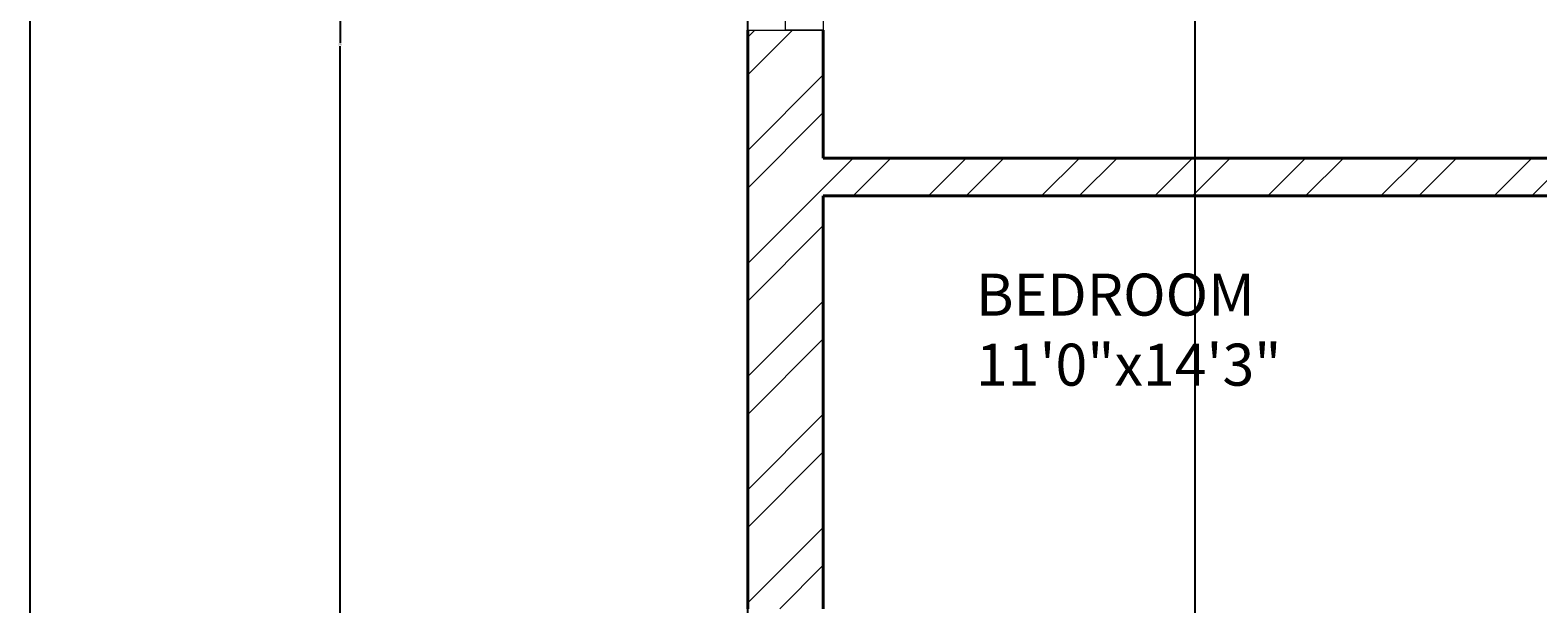
# Model space of a CAD drawing. Units: inches. Extents: x 1601 to 2297, y 1496 to 2631.
# Tile 3 of 57: x 1601 to 1780, y 1767 to 1835. Entities that reach past the tile are written whole.
import ezdxf

# ---------------------------------------------------------------- set-up
doc = ezdxf.new("R2010")
doc.units = ezdxf.units.IN
for name, color, linetype, lineweight in [('A-ANNO-DIMS', 2, 'Continuous', 18), ('A-ANNO-TTLB', 7, 'Continuous', 25), ('A-AREA-IDEN', 7, 'Continuous', 18), ('A-GLAZ', 161, 'Continuous', 20), ('A-WALL', 7, 'Continuous', 40), ('A-WALL-PATT', 215, 'Continuous', 13)]:
    doc.layers.add(name, color=color, linetype=linetype, lineweight=lineweight)
doc.styles.get("Standard").update_dxf_attribs({"font": 'arial.ttf'})
doc.dimstyles.get("Standard").update_dxf_attribs({"dimtxt": 0.18, "dimasz": 0.18, "dimexe": 0.18, "dimexo": 0.0625, "dimgap": 0.09, "dimtad": 0, "dimtih": 1, "dimtoh": 1, "dimdec": 4, "dimzin": 0, "dimdsep": 46, "dimtxsty": 'Standard', "dimcen": 0.09, "dimadec": 0, "dimazin": 0, "dimtfac": 1, "dimtdec": 4, "dimtofl": 0, "dimtmove": 0, "dimatfit": 3, "dimfxl": 1, "dimtolj": 1, "dimtzin": 0, "dimarcsym": 0})

# ---------------------------------------------------------------- blocks, each defined once
blk = doc.blocks.new('WIN-24IN-JAMB9')
for p, q in [((4.5, 24), (0, 24)), ((0, 24), (9, 24)), ((0, 24), (0, 0)), ((4.5, 0), (4.5, 24)), ((9, 24), (9, 0)), ((0, 0), (9, 0)), ((9, 0), (4.5, 0))]:
    blk.add_line(p, q)
blk = doc.blocks.new('*D30')
at = {"layer": 'A-ANNO-DIMS', "color": 0, "lineweight": -2, "transparency": 16777216}
for p, q in [((1685.97, 2031.33), (1637.31, 2031.33)), ((1637.49, 2031.15), (1637.49, 1833.51)), ((1637.49, 1635.51), (1637.49, 1833.14)), ((1685.97, 1635.33), (1637.31, 1635.33))]:
    blk.add_line(p, q, dxfattribs=at)
at = {"layer": 'A-ANNO-DIMS', "color": 0, "transparency": 16777216}
for points in [[(1637.46, 2031.15), (1637.52, 2031.15), (1637.49, 2031.33)], [(1637.46, 1635.51), (1637.52, 1635.51), (1637.49, 1635.33)]]:
    blk.add_solid(points, dxfattribs=at)
at = {"layer": 'Defpoints', "color": 0, "transparency": 16777216}
for p in [(1637.49, 2031.33), (1686.04, 2031.33), (1686.04, 1635.33)]:
    blk.add_point(p, dxfattribs=at)
at = {"layer": 'A-ANNO-DIMS', "color": 0, "transparency": 16777216, "insert": (1637.49, 1833.33), "char_height": 0.18, "attachment_point": 5}
blk.add_mtext('\\A1;396', dxfattribs=at)
blk = doc.blocks.new('*D36')
at = {"layer": 'A-ANNO-DIMS', "color": 0, "lineweight": -2, "transparency": 16777216}
for p, q in [((1686.04, 1635.39), (1686.04, 2581.06)), ((1686.22, 2580.88), (1712.36, 2580.88)), ((1739.15, 2580.88), (1713.01, 2580.88)), ((1739.33, 1635.39), (1739.33, 2581.06))]:
    blk.add_line(p, q, dxfattribs=at)
at = {"layer": 'A-ANNO-DIMS', "color": 0, "transparency": 16777216}
for points in [[(1686.22, 2580.91), (1686.22, 2580.85), (1686.04, 2580.88)], [(1739.15, 2580.91), (1739.15, 2580.85), (1739.33, 2580.88)]]:
    blk.add_solid(points, dxfattribs=at)
at = {"layer": 'Defpoints', "color": 0, "transparency": 16777216}
for p in [(1739.33, 2580.88), (1686.04, 1635.33), (1739.33, 1635.33)]:
    blk.add_point(p, dxfattribs=at)
at = {"layer": 'A-ANNO-DIMS', "color": 0, "transparency": 16777216, "insert": (1712.69, 2580.88), "char_height": 0.18, "attachment_point": 5}
blk.add_mtext('\\A1;53.3', dxfattribs=at)

msp = doc.modelspace()

# ---------------------------------------------------------------- hatches: boundary and pattern name
at = {"layer": 'A-WALL-PATT'}
h = msp.add_hatch(dxfattribs=at)
h.set_pattern_fill('ANSI32', color=256)
h.paths.add_polyline_path([(1842.0336, 2528.0767), (1842.0336, 2532.3254), (1686.0373, 2532.3254), (1686.0373, 2492.9493), (1695.0373, 2492.9493), (1695.0373, 2523.3254), (1827.0373, 2523.3254), (1827.0373, 2416.8254), (1834.6225, 2416.8254), (1834.6225, 2419.0754), (1834.6225, 2421.3254), (1831.5373, 2421.3254), (1831.5373, 2523.3254), (1842.0336, 2523.3254)])
h.paths.add_polyline_path([(1695.0373, 2432.9493), (1686.0373, 2432.9493), (1686.0373, 2325.989), (1695.0373, 2325.989), (1695.0373, 2347.8254), (1827.0373, 2347.8254), (1827.0373, 2287.8254), (1823.2991, 2287.8254), (1823.2991, 2283.3254), (1847.9422, 2283.3254), (1847.9422, 2285.5754), (1847.9422, 2287.8254), (1831.5373, 2287.8254), (1831.5373, 2347.8254), (1846.9946, 2347.8254), (1846.9946, 2350.0754), (1846.9946, 2352.3254), (1695.0373, 2352.3254)])
h.paths.add_polyline_path([(1807.1169, 1573.5395), (2055.0405, 1573.5395), (2055.0405, 1610.6322), (1807.1169, 1610.6322)], flags=9)
h.paths.add_polyline_path([(1841.1631, 1712.7967), (1870.3957, 1712.7967), (1870.3957, 1731.454), (1841.1631, 1731.454)], flags=9)
h.paths.add_polyline_path([(2144.3862, 1772.185), (2191.0233, 1772.185), (2191.0233, 1790.8423), (2144.3862, 1790.8423)], flags=9)
h.paths.add_polyline_path([(2143.0128, 1827.3312), (2177.9958, 1827.3312), (2177.9958, 1845.9886), (2143.0128, 1845.9886)], flags=9)
h.paths.add_polyline_path([(2041.2439, 1833.5691), (2070.8516, 1833.5691), (2070.8516, 1852.2264), (2041.2439, 1852.2264)], flags=9)
h.paths.add_polyline_path([(2097.2791, 1947.0598), (2134.2061, 1947.0598), (2134.2061, 1965.7171), (2097.2791, 1965.7171)], flags=9)
h.paths.add_polyline_path([(2214.995, 1904.3124), (2214.995, 1942.2899), (2196.3376, 1942.2899), (2196.3376, 1904.3124)], flags=9)
h.paths.add_polyline_path([(2186.6284, 2043.8031), (2219.7935, 2043.8031), (2219.7935, 2062.4605), (2186.6284, 2062.4605)], flags=9)
h.paths.add_polyline_path([(2064.0877, 2031.616), (2097.4949, 2031.616), (2097.4949, 2050.2734), (2064.0877, 2050.2734)], flags=9)
h.paths.add_polyline_path([(1973.1349, 1986.0688), (2008.4009, 1986.0688), (2008.4009, 2004.7261), (1973.1349, 2004.7261)], flags=9)
h.paths.add_polyline_path([(1976.3676, 2106.9635), (2005.7469, 2106.9635), (2005.7469, 2125.6209), (1976.3676, 2125.6209)], flags=9)
h.paths.add_polyline_path([(1991.7852, 2180.4863), (2027.0513, 2180.4863), (2027.0513, 2199.1437), (1991.7852, 2199.1437)], flags=9)
h.paths.add_polyline_path([(2106.1801, 2187.9359), (2152.2101, 2187.9359), (2152.2101, 2206.5932), (2106.1801, 2206.5932)], flags=9)
h.paths.add_polyline_path([(2148.6686, 2262.2542), (2182.318, 2262.2542), (2182.318, 2280.9115), (2148.6686, 2280.9115)], flags=9)
h.paths.add_polyline_path([(2041.6327, 2252.8147), (2071.2405, 2252.8147), (2071.2405, 2271.4721), (2041.6327, 2271.4721)], flags=9)
h.paths.add_polyline_path([(2063.9734, 2375.4265), (2100.9004, 2375.4265), (2100.9004, 2394.0839), (2063.9734, 2394.0839)], flags=9)
h.paths.add_polyline_path([(2216.4955, 2330.9748), (2216.4955, 2370.2654), (2197.8381, 2370.2654), (2197.8381, 2330.9748)], flags=9)
h.paths.add_polyline_path([(2179.1416, 2485.8687), (2212.3067, 2485.8687), (2212.3067, 2504.5261), (2179.1416, 2504.5261)], flags=9)
h.paths.add_polyline_path([(2078.7442, 2471.1516), (2112.1514, 2471.1516), (2112.1514, 2489.809), (2078.7442, 2489.809)], flags=9)
h.paths.add_polyline_path([(1915.9631, 2329.4668), (1952.8902, 2329.4668), (1952.8902, 2348.1241), (1915.9631, 2348.1241)], flags=9)
h.paths.add_polyline_path([(1904.3189, 2499.6709), (1940.4512, 2499.6709), (1940.4512, 2518.3282), (1904.3189, 2518.3282)], flags=9)
h.paths.add_polyline_path([(1892.3665, 2100.4595), (1925.6374, 2100.4595), (1925.6374, 2119.1169), (1892.3665, 2119.1169)], flags=9)
h.paths.add_polyline_path([(1909.2984, 1805.9631), (1946.2254, 1805.9631), (1946.2254, 1824.6205), (1909.2984, 1824.6205)], flags=9)
h.paths.add_polyline_path([(1934.6056, 1658.616), (1970.738, 1658.616), (1970.738, 1677.2733), (1934.6056, 1677.2733)], flags=9)
h.paths.add_polyline_path([(1711.2052, 1789.8902), (1750.0456, 1789.8902), (1750.0456, 1808.5476), (1711.2052, 1808.5476)], flags=9)
h.paths.add_polyline_path([(1742.7874, 1854.6743), (1771.9449, 1854.6743), (1771.9449, 1873.3317), (1742.7874, 1873.3317)], flags=9)
h.paths.add_polyline_path([(1807.3592, 1997.7912), (1850.1116, 1997.7912), (1850.1116, 2016.4486), (1807.3592, 2016.4486)], flags=9)
h.paths.add_polyline_path([(1717.4579, 2237.7844), (1760.2103, 2237.7844), (1760.2103, 2256.4417), (1717.4579, 2256.4417)], flags=9)
h.paths.add_polyline_path([(1780.9285, 2324.0623), (1810.086, 2324.0623), (1810.086, 2342.7197), (1780.9285, 2342.7197)], flags=25)
h.paths.add_polyline_path([(1837.696, 2449.2024), (1866.9286, 2449.2024), (1866.9286, 2467.8598), (1837.696, 2467.8598)], flags=9)
h.paths.add_polyline_path([(1712.7752, 2484.9404), (1751.6156, 2484.9404), (1751.6156, 2503.5977), (1712.7752, 2503.5977)], flags=25)
h = msp.add_hatch(dxfattribs=at)
h.set_pattern_fill('ANSI32', color=256)
h.paths.add_polyline_path([(1973.9371, 2211.3254), (1893.0373, 2211.3254), (1893.0373, 2287.8254), (1884.6167, 2287.8254), (1884.6167, 2285.5754), (1884.6167, 2283.3254), (1888.5373, 2283.3254), (1888.5373, 2145.3254), (1695.0373, 2145.3254), (1695.0373, 2173.8724), (1690.5373, 2173.8724), (1686.0373, 2173.8724), (1686.0373, 2136.3254), (1722.5687, 2136.3254), (1722.5687, 2117.4352), (1731.5687, 2117.4352), (1731.5687, 2136.3254), (1893.0373, 2136.3254), (1893.0373, 2202.3254), (1959.0373, 2202.3254), (1959.0373, 2182.1303), (1968.0373, 2182.1303), (1968.0373, 2202.3254), (1973.9371, 2202.3254)])
h.paths.add_polyline_path([(2094.0373, 2274.6364), (2096.4294, 2274.6364), (2096.4294, 2276.8864), (2096.4294, 2279.1364), (2094.0373, 2279.1364), (2094.0373, 2290.8254), (2094.0373, 2295.3254), (2089.5373, 2295.3254), (2089.5373, 2230.8254), (2035.5373, 2230.8254), (2035.5373, 2299.8254), (2031.0373, 2299.8254), (2031.0373, 2211.3254), (2023.0065, 2211.3254), (2023.0065, 2202.3254), (2031.0373, 2202.3254), (2031.0373, 2140.8254), (1968.0373, 2140.8254), (1968.0373, 2145.9106), (1963.5373, 2145.9106), (1959.0373, 2145.9106), (1959.0373, 2116.839), (1963.5373, 2116.839), (1968.0373, 2116.839), (1968.0373, 2131.8254), (2031.0373, 2131.8254), (2031.0373, 2094.3254), (2031.0373, 2085.3254), (2031.0373, 2056.8254), (1968.0373, 2056.8254), (1968.0373, 2070.4947), (1963.5373, 2070.4947), (1959.0373, 2070.4947), (1959.0373, 2040.3029), (1968.0373, 2040.3029), (1968.0373, 2047.8254), (2031.0373, 2047.8254), (2031.0373, 1983.3254), (2031.0373, 1978.8254), (2021.1979, 1978.8254), (2021.1979, 1974.3254), (2031.0373, 1974.3254), (2031.0373, 1954.3528), (2035.5373, 1954.3528), (2035.5373, 1974.3254), (2035.5373, 1981.8254), (2055.5513, 1981.8254), (2055.5513, 1986.3254), (2035.5373, 1986.3254), (2035.5373, 2047.8254), (2040.0373, 2047.8254), (2040.0373, 2085.3254), (2040.0373, 2094.3254), (2040.0373, 2140.8254), (2035.5373, 2140.8254), (2035.5373, 2226.3254), (2089.5373, 2226.3254), (2094.0373, 2226.3254)])
h.paths.add_polyline_path([(2226.0373, 2230.8254), (2134.5373, 2230.8254), (2134.5373, 2233.5437), (2130.0373, 2233.5437), (2130.0373, 2226.3254), (2134.5373, 2226.3254), (2226.0373, 2226.3254)])
h.paths.add_polyline_path([(1807.1169, 1573.5395), (2055.0405, 1573.5395), (2055.0405, 1610.6322), (1807.1169, 1610.6322)], flags=9)
h.paths.add_polyline_path([(1841.1631, 1712.7967), (1870.3957, 1712.7967), (1870.3957, 1731.454), (1841.1631, 1731.454)], flags=9)
h.paths.add_polyline_path([(2144.3862, 1772.185), (2191.0233, 1772.185), (2191.0233, 1790.8423), (2144.3862, 1790.8423)], flags=9)
h.paths.add_polyline_path([(2143.0128, 1827.3312), (2177.9958, 1827.3312), (2177.9958, 1845.9886), (2143.0128, 1845.9886)], flags=9)
h.paths.add_polyline_path([(2041.2439, 1833.5691), (2070.8516, 1833.5691), (2070.8516, 1852.2264), (2041.2439, 1852.2264)], flags=9)
h.paths.add_polyline_path([(2097.2791, 1947.0598), (2134.2061, 1947.0598), (2134.2061, 1965.7171), (2097.2791, 1965.7171)], flags=9)
h.paths.add_polyline_path([(2214.995, 1904.3124), (2214.995, 1942.2899), (2196.3376, 1942.2899), (2196.3376, 1904.3124)], flags=9)
h.paths.add_polyline_path([(2186.6284, 2043.8031), (2219.7935, 2043.8031), (2219.7935, 2062.4605), (2186.6284, 2062.4605)], flags=9)
h.paths.add_polyline_path([(2064.0877, 2031.616), (2097.4949, 2031.616), (2097.4949, 2050.2734), (2064.0877, 2050.2734)], flags=9)
h.paths.add_polyline_path([(1973.1349, 1986.0688), (2008.4009, 1986.0688), (2008.4009, 2004.7261), (1973.1349, 2004.7261)], flags=25)
h.paths.add_polyline_path([(1976.3676, 2106.9635), (2005.7469, 2106.9635), (2005.7469, 2125.6209), (1976.3676, 2125.6209)], flags=25)
h.paths.add_polyline_path([(1991.7852, 2180.4863), (2027.0513, 2180.4863), (2027.0513, 2199.1437), (1991.7852, 2199.1437)], flags=25)
h.paths.add_polyline_path([(2106.1801, 2187.9359), (2152.2101, 2187.9359), (2152.2101, 2206.5932), (2106.1801, 2206.5932)], flags=9)
h.paths.add_polyline_path([(2148.6686, 2262.2542), (2182.318, 2262.2542), (2182.318, 2280.9115), (2148.6686, 2280.9115)], flags=9)
h.paths.add_polyline_path([(2041.6327, 2252.8147), (2071.2405, 2252.8147), (2071.2405, 2271.4721), (2041.6327, 2271.4721)], flags=25)
h.paths.add_polyline_path([(2063.9734, 2375.4265), (2100.9004, 2375.4265), (2100.9004, 2394.0839), (2063.9734, 2394.0839)], flags=9)
h.paths.add_polyline_path([(2216.4955, 2330.9748), (2216.4955, 2370.2654), (2197.8381, 2370.2654), (2197.8381, 2330.9748)], flags=9)
h.paths.add_polyline_path([(2179.1416, 2485.8687), (2212.3067, 2485.8687), (2212.3067, 2504.5261), (2179.1416, 2504.5261)], flags=9)
h.paths.add_polyline_path([(2078.7442, 2471.1516), (2112.1514, 2471.1516), (2112.1514, 2489.809), (2078.7442, 2489.809)], flags=9)
h.paths.add_polyline_path([(1915.9631, 2329.4668), (1952.8902, 2329.4668), (1952.8902, 2348.1241), (1915.9631, 2348.1241)], flags=9)
h.paths.add_polyline_path([(1904.3189, 2499.6709), (1940.4512, 2499.6709), (1940.4512, 2518.3282), (1904.3189, 2518.3282)], flags=9)
h.paths.add_polyline_path([(1892.3665, 2100.4595), (1925.6374, 2100.4595), (1925.6374, 2119.1169), (1892.3665, 2119.1169)], flags=9)
h.paths.add_polyline_path([(1909.2984, 1805.9631), (1946.2254, 1805.9631), (1946.2254, 1824.6205), (1909.2984, 1824.6205)], flags=9)
h.paths.add_polyline_path([(1934.6056, 1658.616), (1970.738, 1658.616), (1970.738, 1677.2733), (1934.6056, 1677.2733)], flags=9)
h.paths.add_polyline_path([(1711.2052, 1789.8902), (1750.0456, 1789.8902), (1750.0456, 1808.5476), (1711.2052, 1808.5476)], flags=9)
h.paths.add_polyline_path([(1742.7874, 1854.6743), (1771.9449, 1854.6743), (1771.9449, 1873.3317), (1742.7874, 1873.3317)], flags=9)
h.paths.add_polyline_path([(1807.3592, 1997.7912), (1850.1116, 1997.7912), (1850.1116, 2016.4486), (1807.3592, 2016.4486)], flags=9)
h.paths.add_polyline_path([(1717.4579, 2237.7844), (1760.2103, 2237.7844), (1760.2103, 2256.4417), (1717.4579, 2256.4417)], flags=25)
h.paths.add_polyline_path([(1780.9285, 2324.0623), (1810.086, 2324.0623), (1810.086, 2342.7197), (1780.9285, 2342.7197)], flags=9)
h.paths.add_polyline_path([(1837.696, 2449.2024), (1866.9286, 2449.2024), (1866.9286, 2467.8598), (1837.696, 2467.8598)], flags=9)
h.paths.add_polyline_path([(1712.7752, 2484.9404), (1751.6156, 2484.9404), (1751.6156, 2503.5977), (1712.7752, 2503.5977)], flags=9)
h = msp.add_hatch(dxfattribs=at)
h.set_pattern_fill('ANSI32', color=256)
h.paths.add_polyline_path([(2230.5373, 1861.8254), (2182.5373, 1861.8254), (2182.5373, 1885.3637), (2178.0373, 1885.3637), (2178.0373, 1861.8254), (2166.0373, 1861.8254), (2134.5373, 1861.8254), (2130.0373, 1861.8254), (2130.0373, 1841.4682), (2126.8833, 1841.4682), (2126.8833, 1836.9682), (2130.0373, 1836.9682), (2130.0373, 1822.7302), (2134.5373, 1822.7302), (2134.5373, 1857.3254), (2166.0373, 1857.3254), (2226.0373, 1857.3254), (2226.0373, 1846.1155), (2230.5373, 1846.1155)])
h.paths.add_polyline_path([(2226.0373, 1797.3254), (2134.5373, 1797.3254), (2134.5373, 1800.6636), (2132.2873, 1800.6636), (2130.0373, 1800.6636), (2130.0373, 1797.3254), (2130.0373, 1792.8254), (2167.7264, 1792.8254), (2226.0373, 1792.8254)])
h.paths.add_polyline_path([(2230.5373, 1822.1155), (2226.0373, 1822.1155), (2226.0373, 1760.8563), (2230.5373, 1760.8563)])
h.paths.add_polyline_path([(2230.5373, 1700.8563), (2226.0373, 1700.8563), (2226.0373, 1644.3254), (2140.2517, 1644.3254), (2140.2517, 1635.3254), (2230.5373, 1635.3254)])
h.paths.add_polyline_path([(2080.2517, 1639.8254), (2080.2517, 1644.3254), (2035.5373, 1644.3254), (2035.5373, 1792.8254), (2094.0373, 1792.8254), (2094.0373, 1797.3254), (2094.0373, 1836.9682), (2097.1057, 1836.9682), (2097.1057, 1839.2182), (2097.1057, 1841.4682), (2094.0373, 1841.4682), (2094.0373, 1862.2276), (2089.5373, 1862.2276), (2089.5373, 1797.3254), (2035.5373, 1797.3254), (2035.5373, 1857.3254), (2035.5373, 1885.0916), (2031.0373, 1885.0916), (2031.0373, 1710.3254), (2012.329, 1710.3254), (2012.329, 1701.3254), (2031.0373, 1701.3254), (2031.0373, 1644.3254), (2031.0373, 1635.3254), (2080.2517, 1635.3254)])
h.paths.add_polyline_path([(1836.0373, 1653.2033), (1842.6171, 1653.2033), (1842.6171, 1657.7033), (1842.6171, 1662.2033), (1831.5373, 1662.2033), (1831.5373, 1764.2033), (1835.3881, 1764.2033), (1835.3881, 1766.4533), (1835.3881, 1768.7033), (1831.5373, 1768.7033), (1827.0373, 1768.7033), (1827.0373, 1662.2033), (1827.0373, 1635.3254), (1836.0373, 1635.3254)])
h.paths.add_polyline_path([(1893.0373, 1701.3254), (1907.193, 1701.3254), (1907.193, 1705.8254), (1907.193, 1710.3254), (1893.0373, 1710.3254), (1893.0373, 1819.8254), (1882.6444, 1819.8254), (1882.6444, 1817.5754), (1882.6444, 1815.3254), (1888.5373, 1815.3254), (1888.5373, 1662.2033), (1884.0373, 1662.2033), (1866.6171, 1662.2033), (1866.6171, 1653.2033), (1882.391, 1653.2033), (1884.0373, 1653.2033), (1884.0373, 1635.3254), (1893.0373, 1635.3254)])
h.paths.add_polyline_path([(1739.3335, 1639.8254), (1739.3335, 1644.3254), (1695.0373, 1644.3254), (1695.0373, 1702.0135), (1690.5373, 1702.0135), (1686.0373, 1702.0135), (1686.0373, 1635.3254), (1739.3335, 1635.3254)])
h.paths.add_polyline_path([(1827.0373, 1644.3254), (1799.3335, 1644.3254), (1799.3335, 1635.3254), (1827.0373, 1635.3254)])
h.paths.add_polyline_path([(1695.0373, 1815.3254), (1849.2759, 1815.3254), (1849.2759, 1819.8254), (1807.5373, 1819.8254), (1807.5373, 1879.8254), (1851.1533, 1879.8254), (1851.1533, 1882.0754), (1851.1533, 1884.3254), (1799.3405, 1884.3254), (1799.3405, 1882.0754), (1799.3405, 1879.8254), (1803.0373, 1879.8254), (1803.0373, 1819.8254), (1695.0373, 1819.8254), (1695.0373, 1835.0458), (1690.5373, 1835.0458), (1686.0373, 1835.0458), (1686.0373, 1766.1753), (1695.0373, 1766.1753)])
h.paths.add_polyline_path([(1775.8157, 1884.3254), (1695.0373, 1884.3254), (1695.0373, 1912.9526), (1690.5373, 1912.9526), (1686.0373, 1912.9526), (1686.0373, 1859.0458), (1695.0373, 1859.0458), (1695.0373, 1879.8254), (1775.8157, 1879.8254)])
h.paths.add_polyline_path([(1893.0373, 2031.3254), (1731.5687, 2031.3254), (1731.5687, 2057.4352), (1722.5687, 2057.4352), (1722.5687, 2031.3254), (1686.0373, 2031.3254), (1686.0373, 1972.9526), (1695.0373, 1972.9526), (1695.0373, 2022.3254), (1888.5373, 2022.3254), (1888.5373, 1884.3254), (1883.4996, 1884.3254), (1883.4996, 1879.8254), (1893.0373, 1879.8254), (1893.0373, 1974.3254), (1976.6199, 1974.3254), (1976.6199, 1978.8254), (1968.0373, 1978.8254), (1968.0373, 1983.3254), (1968.0373, 2008.4756), (1963.5373, 2008.4756), (1959.0373, 2008.4756), (1959.0373, 1983.3254), (1893.0373, 1983.3254)])
h.paths.add_polyline_path([(2230.5373, 2140.4745), (2226.0373, 2140.4745), (2226.0373, 2094.3254), (2040.0373, 2094.3254), (2040.0373, 2085.3254), (2178.0373, 2085.3254), (2178.0373, 2065.6965), (2182.5373, 2065.6965), (2182.5373, 2085.3254), (2226.0373, 2085.3254), (2226.0373, 1986.3254), (2211.2679, 1986.3254), (2211.2679, 1981.8254), (2230.5373, 1981.8254)])
h.paths.add_polyline_path([(2187.6292, 1986.3254), (2182.5373, 1986.3254), (2182.5373, 2029.6965), (2178.0373, 2029.6965), (2178.0373, 1986.3254), (2099.05, 1986.3254), (2099.05, 1981.8254), (2178.0373, 1981.8254), (2178.0373, 1969.3637), (2182.5373, 1969.3637), (2182.5373, 1981.8254), (2187.6292, 1981.8254), (2187.6292, 1984.0754)])
h.paths.add_polyline_path([(1807.1169, 1573.5395), (2055.0405, 1573.5395), (2055.0405, 1610.6322), (1807.1169, 1610.6322)], flags=9)
h.paths.add_polyline_path([(1841.1631, 1712.7967), (1870.3957, 1712.7967), (1870.3957, 1731.454), (1841.1631, 1731.454)], flags=9)
h.paths.add_polyline_path([(2144.3862, 1772.185), (2191.0233, 1772.185), (2191.0233, 1790.8423), (2144.3862, 1790.8423)], flags=9)
h.paths.add_polyline_path([(2143.0128, 1827.3312), (2177.9958, 1827.3312), (2177.9958, 1845.9886), (2143.0128, 1845.9886)], flags=25)
h.paths.add_polyline_path([(2041.2439, 1833.5691), (2070.8516, 1833.5691), (2070.8516, 1852.2264), (2041.2439, 1852.2264)], flags=25)
h.paths.add_polyline_path([(2097.2791, 1947.0598), (2134.2061, 1947.0598), (2134.2061, 1965.7171), (2097.2791, 1965.7171)], flags=9)
h.paths.add_polyline_path([(2214.995, 1904.3124), (2214.995, 1942.2899), (2196.3376, 1942.2899), (2196.3376, 1904.3124)], flags=9)
h.paths.add_polyline_path([(2186.6284, 2043.8031), (2219.7935, 2043.8031), (2219.7935, 2062.4605), (2186.6284, 2062.4605)], flags=25)
h.paths.add_polyline_path([(2064.0877, 2031.616), (2097.4949, 2031.616), (2097.4949, 2050.2734), (2064.0877, 2050.2734)], flags=25)
h.paths.add_polyline_path([(1973.1349, 1986.0688), (2008.4009, 1986.0688), (2008.4009, 2004.7261), (1973.1349, 2004.7261)], flags=9)
h.paths.add_polyline_path([(1976.3676, 2106.9635), (2005.7469, 2106.9635), (2005.7469, 2125.6209), (1976.3676, 2125.6209)], flags=9)
h.paths.add_polyline_path([(1991.7852, 2180.4863), (2027.0513, 2180.4863), (2027.0513, 2199.1437), (1991.7852, 2199.1437)], flags=9)
h.paths.add_polyline_path([(2106.1801, 2187.9359), (2152.2101, 2187.9359), (2152.2101, 2206.5932), (2106.1801, 2206.5932)], flags=9)
h.paths.add_polyline_path([(2148.6686, 2262.2542), (2182.318, 2262.2542), (2182.318, 2280.9115), (2148.6686, 2280.9115)], flags=9)
h.paths.add_polyline_path([(2041.6327, 2252.8147), (2071.2405, 2252.8147), (2071.2405, 2271.4721), (2041.6327, 2271.4721)], flags=9)
h.paths.add_polyline_path([(2063.9734, 2375.4265), (2100.9004, 2375.4265), (2100.9004, 2394.0839), (2063.9734, 2394.0839)], flags=9)
h.paths.add_polyline_path([(2216.4955, 2330.9748), (2216.4955, 2370.2654), (2197.8381, 2370.2654), (2197.8381, 2330.9748)], flags=9)
h.paths.add_polyline_path([(2179.1416, 2485.8687), (2212.3067, 2485.8687), (2212.3067, 2504.5261), (2179.1416, 2504.5261)], flags=9)
h.paths.add_polyline_path([(2078.7442, 2471.1516), (2112.1514, 2471.1516), (2112.1514, 2489.809), (2078.7442, 2489.809)], flags=9)
h.paths.add_polyline_path([(1915.9631, 2329.4668), (1952.8902, 2329.4668), (1952.8902, 2348.1241), (1915.9631, 2348.1241)], flags=9)
h.paths.add_polyline_path([(1904.3189, 2499.6709), (1940.4512, 2499.6709), (1940.4512, 2518.3282), (1904.3189, 2518.3282)], flags=9)
h.paths.add_polyline_path([(1892.3665, 2100.4595), (1925.6374, 2100.4595), (1925.6374, 2119.1169), (1892.3665, 2119.1169)], flags=9)
h.paths.add_polyline_path([(1909.2984, 1805.9631), (1946.2254, 1805.9631), (1946.2254, 1824.6205), (1909.2984, 1824.6205)], flags=9)
h.paths.add_polyline_path([(1934.6056, 1658.616), (1970.738, 1658.616), (1970.738, 1677.2733), (1934.6056, 1677.2733)], flags=9)
h.paths.add_polyline_path([(1711.2052, 1789.8902), (1750.0456, 1789.8902), (1750.0456, 1808.5476), (1711.2052, 1808.5476)], flags=25)
h.paths.add_polyline_path([(1742.7874, 1854.6743), (1771.9449, 1854.6743), (1771.9449, 1873.3317), (1742.7874, 1873.3317)], flags=25)
h.paths.add_polyline_path([(1807.3592, 1997.7912), (1850.1116, 1997.7912), (1850.1116, 2016.4486), (1807.3592, 2016.4486)], flags=25)
h.paths.add_polyline_path([(1717.4579, 2237.7844), (1760.2103, 2237.7844), (1760.2103, 2256.4417), (1717.4579, 2256.4417)], flags=9)
h.paths.add_polyline_path([(1780.9285, 2324.0623), (1810.086, 2324.0623), (1810.086, 2342.7197), (1780.9285, 2342.7197)], flags=9)
h.paths.add_polyline_path([(1837.696, 2449.2024), (1866.9286, 2449.2024), (1866.9286, 2467.8598), (1837.696, 2467.8598)], flags=9)
h.paths.add_polyline_path([(1712.7752, 2484.9404), (1751.6156, 2484.9404), (1751.6156, 2503.5977), (1712.7752, 2503.5977)], flags=9)

# ---------------------------------------------------------------- linework, layer by layer
at = {"layer": 'A-ANNO-TTLB'}
msp.add_lwpolyline([(1600.5933, 2631.1477), (2297.129, 2631.1477), (2297.129, 1496.1026), (1600.5933, 1496.1026)], close=True, dxfattribs=at)
at = {"layer": 'A-WALL'}
for p, q in [((1686.0373, 1835.0458), (1686.0373, 1766.1753)), ((1695.0373, 1835.0458), (1695.0373, 1819.8254)), ((1695.0373, 1819.8254), (1803.0373, 1819.8254)), ((1695.0373, 1815.3254), (1850.9031, 1815.3254)), ((1695.0373, 1815.3254), (1695.0373, 1766.1753))]:
    msp.add_line(p, q, dxfattribs=at)

# ---------------------------------------------------------------- block references
at = {"layer": 'A-GLAZ'}
msp.add_blockref('WIN-24IN-JAMB9', (1686.037, 1835.046), dxfattribs=at)

# ---------------------------------------------------------------- texts
at = {"layer": 'A-AREA-IDEN', "insert": (1713.2157, 1806.0629), "char_height": 5, "attachment_point": 1}
msp.add_mtext_dynamic_manual_height_columns('BEDROOM\\P11\'0"x14\'3"', width=135.852725, gutter_width=12.5, heights=[0], dxfattribs=at)

# ---------------------------------------------------------------- dimensions: what is measured, and where the dimension line sits
at = {"layer": 'A-ANNO-DIMS'}
dim = msp.add_linear_dim(base=(1739.3335, 2580.8754), p1=(1686.0373, 1635.3254), p2=(1739.3335, 1635.3254), dimstyle='Standard', override={"dimdec": 1, "dimlfac": 1, "dimrnd": 0, "dimzin": 0, "dimdsep": 46, "dimlunit": 2}, dxfattribs=at)
dim.commit()
dim.dimension.update_dxf_attribs({"geometry": '*D36', "text_midpoint": (1712.6854, 2580.8754)})
dim = msp.add_linear_dim(base=(1637.4873, 2031.3254), p1=(1686.0373, 1635.3254), p2=(1686.0373, 2031.3254), angle=90, dimstyle='Standard', override={"dimdec": 0, "dimlfac": 1, "dimrnd": 0, "dimzin": 0, "dimdsep": 46, "dimlunit": 2}, dxfattribs=at)
dim.commit()
dim.dimension.update_dxf_attribs({"geometry": '*D30', "text_midpoint": (1637.4873, 1833.3254)})

doc.saveas('drawing.dxf')
